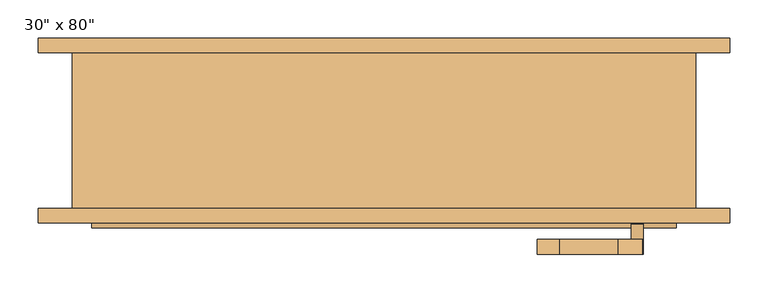
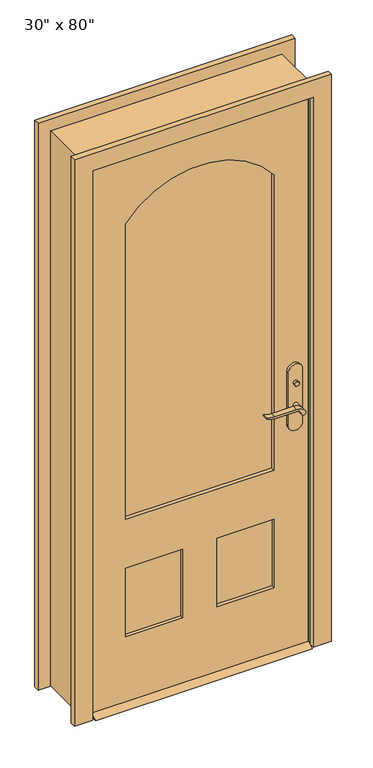
"""IFC4 building model written with IfcOpenShell, lengths in millimetres: door geometry."""

from ifc_helpers import new_model, si_unit, point, frame, frame_2d, origin, place, context, project, spatial, polyline, circle_curve, trimmed, segment, composite_curve, outline, extrude, faceted_brep, source, transform, mapped, element, save


def door_41326d50(model_context):
    return source(origin(), model_context, "Body", "SolidModel", [
        extrude(outline(polyline([(-63.5, 12.7), (-38.1, 0.0), (-123.825, 0.0), (-98.425, 12.7), (-63.5, 12.7)])), frame((-381.0, 0.0, 0.0), z_axis=(1.0, 0.0, 0.0), x_axis=(0.0, 1.0, 0.0)), (0.0, 0.0, 1.0), 762.0),
        extrude(outline(polyline([(335.2, -43.5), (335.2, -53.5), (325.2, -53.5), (325.2, -43.5), (335.2, -43.5)])), frame((0.0, 0.0, 981.9), z_axis=(0.0, 0.0, 1.0), x_axis=(1.0, 0.0, 0.0)), (0.0, 0.0, 1.0), 30.0),
        extrude(outline(composite_curve([segment(trimmed(circle_curve(frame_2d((996.9, 330.2)), 8.0), [point((996.9, 322.2))], [point((996.9, 338.2))], False, "CARTESIAN"), True, "CONTINUOUS"), segment(trimmed(circle_curve(frame_2d((996.9, 330.2)), 8.0), [point((996.9, 338.2))], [point((996.9, 322.2))], False, "CARTESIAN"), True, "CONTINUOUS")], self_intersect=False)), frame((0.0, -118.425, 0.0), z_axis=(0.0, 1.0, 0.0), x_axis=(0.0, 0.0, 1.0)), (0.0, 0.0, 1.0), 10.0),
        extrude(outline(composite_curve([segment(trimmed(circle_curve(frame_2d((897.1555521, 306.5324871)), 37.2832219), [point((919.0523287, 336.7081363))], [point((934.4, 304.8325667))], False, "CARTESIAN"), True, "CONTINUOUS"), segment(polyline([(934.4, 304.8325667), (934.4, 228.5564091)]), True, "CONTINUOUS"), segment(trimmed(circle_curve(frame_2d((1017.6850638, 228.6227909)), 83.2850902), [point((934.4, 228.5564091))], [point((939.4, 200.2))], True, "CARTESIAN"), True, "CONTINUOUS"), segment(polyline([(939.4, 200.2), (936.6135558, 200.2)]), True, "CONTINUOUS"), segment(trimmed(circle_curve(frame_2d((986.6709207, 232.1396612)), 59.3791355), [point((936.6135558, 200.2))], [point((927.4, 228.5564091))], False, "CARTESIAN"), True, "CONTINUOUS"), segment(polyline([(927.4, 228.5564091), (927.4, 304.8138099)]), True, "CONTINUOUS"), segment(trimmed(circle_curve(frame_2d((909.2738613, 304.8138099)), 18.1261387), [point((927.4, 304.8138099))], [point((914.4, 322.2))], True, "CARTESIAN"), True, "CONTINUOUS"), segment(trimmed(circle_curve(frame_2d((914.4, 330.2)), 8.0), [point((914.4, 322.2))], [point((919.0523287, 336.7081363))], False, "CARTESIAN"), True, "CONTINUOUS")], self_intersect=False)), frame((0.0, -23.5, 0.0), z_axis=(0.0, 1.0, 0.0), x_axis=(0.0, 0.0, 1.0)), (0.0, 0.0, 1.0), 20.0),
        extrude(outline(composite_curve([segment(trimmed(circle_curve(frame_2d((914.4, 330.2)), 8.0), [point((914.3999903, 322.2))], [point((919.0523287, 336.7081363))], False, "CARTESIAN"), True, "CONTINUOUS"), segment(trimmed(circle_curve(frame_2d((897.1555521, 306.5324871)), 37.2832219), [point((919.0523287, 336.7081363))], [point((934.4, 304.8325667))], False, "CARTESIAN"), True, "CONTINUOUS"), segment(polyline([(934.4, 304.8325667), (934.4, 228.5564091)]), True, "CONTINUOUS"), segment(trimmed(circle_curve(frame_2d((1017.6850638, 228.6227909)), 83.2850902), [point((934.4, 228.5564091))], [point((939.4, 200.2))], True, "CARTESIAN"), True, "CONTINUOUS"), segment(polyline([(939.4, 200.2), (936.6135558, 200.2)]), True, "CONTINUOUS"), segment(trimmed(circle_curve(frame_2d((986.6709207, 232.1396612)), 59.3791355), [point((936.6135558, 200.2))], [point((927.4, 228.5564091))], False, "CARTESIAN"), True, "CONTINUOUS"), segment(polyline([(927.4, 228.5564091), (927.4, 304.8138122)]), True, "CONTINUOUS"), segment(trimmed(circle_curve(frame_2d((909.2738682, 304.8138122)), 18.1261318), [point((927.4, 304.8138122))], [point((914.3999903, 322.2))], True, "CARTESIAN"), True, "CONTINUOUS")], self_intersect=False)), frame((0.0, -158.425, 0.0), z_axis=(0.0, 1.0, 0.0), x_axis=(0.0, 0.0, 1.0)), (0.0, 0.0, 1.0), 20.0),
        extrude(outline(composite_curve([segment(trimmed(circle_curve(frame_2d((914.4, 330.2)), 8.0), [point((914.4, 322.2))], [point((914.4, 338.2))], False, "CARTESIAN"), True, "CONTINUOUS"), segment(trimmed(circle_curve(frame_2d((914.4, 330.2)), 8.0), [point((914.4, 338.2))], [point((914.4, 322.2))], False, "CARTESIAN"), True, "CONTINUOUS")], self_intersect=False)), frame((0.0, -53.5, 0.0), z_axis=(0.0, 1.0, 0.0), x_axis=(0.0, 0.0, 1.0)), (0.0, 0.0, 1.0), 30.0),
        extrude(outline(composite_curve([segment(trimmed(circle_curve(frame_2d((914.4, 330.2)), 8.0), [point((914.4, 322.2))], [point((914.4, 338.2))], False, "CARTESIAN"), True, "CONTINUOUS"), segment(trimmed(circle_curve(frame_2d((914.4, 330.2)), 8.0), [point((914.4, 338.2))], [point((914.4, 322.2))], False, "CARTESIAN"), True, "CONTINUOUS")], self_intersect=False)), frame((0.0, -138.425, 0.0), z_axis=(0.0, 1.0, 0.0), x_axis=(0.0, 0.0, 1.0)), (0.0, 0.0, 1.0), 30.0),
        extrude(outline(composite_curve([segment(polyline([(844.4, 355.2), (1039.4, 355.2)]), True, "CONTINUOUS"), segment(trimmed(circle_curve(frame_2d((1039.4, 330.2)), 25.0), [point((1039.4, 355.2))], [point((1039.4, 305.2))], False, "CARTESIAN"), True, "CONTINUOUS"), segment(polyline([(1039.4, 305.2), (844.4, 305.2)]), True, "CONTINUOUS"), segment(trimmed(circle_curve(frame_2d((844.4, 330.2)), 25.0), [point((844.4, 305.2))], [point((844.4, 355.2))], False, "CARTESIAN"), True, "CONTINUOUS")], self_intersect=False)), frame((0.0, -63.5, 0.0), z_axis=(0.0, 1.0, 0.0), x_axis=(0.0, 0.0, 1.0)), (0.0, 0.0, 1.0), 10.0),
        extrude(outline(composite_curve([segment(polyline([(844.4, 355.2), (1039.4, 355.2)]), True, "CONTINUOUS"), segment(trimmed(circle_curve(frame_2d((1039.4, 330.2)), 25.0), [point((1039.4, 355.2))], [point((1039.4, 305.2))], False, "CARTESIAN"), True, "CONTINUOUS"), segment(polyline([(1039.4, 305.2), (844.4, 305.2)]), True, "CONTINUOUS"), segment(trimmed(circle_curve(frame_2d((844.4, 330.2)), 25.0), [point((844.4, 305.2))], [point((844.4, 355.2))], False, "CARTESIAN"), True, "CONTINUOUS")], self_intersect=False)), frame((0.0, -108.425, 0.0), z_axis=(0.0, 1.0, 0.0), x_axis=(0.0, 0.0, 1.0)), (0.0, 0.0, 1.0), 10.0),
        extrude(outline(polyline([(2032.0, -381.0), (12.7, -381.0), (12.7, 381.0), (2032.0, 381.0), (2032.0, -381.0)]), holes=[composite_curve([segment(polyline([(688.975, -260.35), (1784.35, -260.35)]), True, "CONTINUOUS"), segment(trimmed(circle_curve(frame_2d((1580.99125, 0.0)), 330.35875), [point((1784.35, -260.35))], [point((1784.35, 260.35))], True, "CARTESIAN"), True, "CONTINUOUS"), segment(polyline([(1784.35, 260.35), (688.975, 260.35), (688.975, -260.35)]), True, "CONTINUOUS")], self_intersect=False), polyline([(508.0, -60.325), (254.0, -60.325), (254.0, -260.35), (508.0, -260.35), (508.0, -60.325)]), polyline([(508.0, 260.35), (254.0, 260.35), (254.0, 60.325), (508.0, 60.325), (508.0, 260.35)])]), frame((0.0, -98.425, 0.0), z_axis=(0.0, 1.0, 0.0), x_axis=(0.0, 0.0, 1.0)), (0.0, 0.0, 1.0), 34.925),
        faceted_brep([(406.4, -98.425, 0.0), (381.0, -98.425, 0.0), (381.0, -63.5, 0.0), (368.3, -63.5, 0.0), (368.3, -28.575, 0.0), (381.0, -28.575, 0.0), (381.0, 104.775, 0.0), (406.4, 104.775, 0.0), (406.4, 104.775, 2057.4), (406.4, -98.425, 2057.4), (381.0, 104.775, 2032.0), (-381.0, 104.775, 2032.0), (-381.0, 104.775, 0.0), (-406.4, 104.775, 0.0), (-406.4, 104.775, 2057.4), (381.0, -28.575, 2032.0), (368.3, -28.575, 2019.3), (-368.3, -28.575, 2019.3), (-368.3, -28.575, 0.0), (-381.0, -28.575, 0.0), (-381.0, -28.575, 2032.0), (368.3, -63.5, 2019.3), (381.0, -63.5, 2032.0), (-381.0, -63.5, 2032.0), (-381.0, -63.5, 0.0), (-368.3, -63.5, 0.0), (-368.3, -63.5, 2019.3), (381.0, -98.425, 2032.0), (-406.4, -98.425, 2057.4), (-406.4, -98.425, 0.0), (-381.0, -98.425, 0.0), (-381.0, -98.425, 2032.0)], [[[0, 1, 2, 3, 4, 5, 6, 7]], [[7, 8, 9, 0]], [[6, 10, 11, 12, 13, 14, 8, 7]], [[5, 15, 10, 6]], [[4, 16, 17, 18, 19, 20, 15, 5]], [[3, 21, 16, 4]], [[2, 22, 23, 24, 25, 26, 21, 3]], [[1, 27, 22, 2]], [[0, 9, 28, 29, 30, 31, 27, 1]], [[8, 14, 28, 9]], [[15, 20, 11, 10]], [[21, 26, 17, 16]], [[27, 31, 23, 22]], [[29, 13, 12, 19, 18, 25, 24, 30]], [[14, 13, 29, 28]], [[20, 19, 12, 11]], [[26, 25, 18, 17]], [[31, 30, 24, 23]]]),
        extrude(outline(polyline([(-60.325, -75.1416667), (-60.325, -86.7833333), (-260.35, -86.7833333), (-260.35, -75.1416667), (-60.325, -75.1416667)])), frame((0.0, 0.0, 254.0), z_axis=(0.0, 0.0, 1.0), x_axis=(1.0, 0.0, 0.0)), (0.0, 0.0, 1.0), 254.0),
        extrude(outline(polyline([(260.35, -75.1416667), (260.35, -86.7833333), (60.325, -86.7833333), (60.325, -75.1416667), (260.35, -75.1416667)])), frame((0.0, 0.0, 254.0), z_axis=(0.0, 0.0, 1.0), x_axis=(1.0, 0.0, 0.0)), (0.0, 0.0, 1.0), 254.0),
        extrude(outline(composite_curve([segment(polyline([(688.975, -260.35), (688.975, 260.35), (1784.35, 260.35)]), True, "CONTINUOUS"), segment(trimmed(circle_curve(frame_2d((1580.99125, 0.0)), 330.35875), [point((1784.35, 260.35))], [point((1784.35, -260.35))], False, "CARTESIAN"), True, "CONTINUOUS"), segment(polyline([(1784.35, -260.35), (688.975, -260.35)]), True, "CONTINUOUS")], self_intersect=False)), frame((0.0, -84.455, 0.0), z_axis=(0.0, 1.0, 0.0), x_axis=(0.0, 0.0, 1.0)), (0.0, 0.0, 1.0), 6.985),
        extrude(outline(polyline([(0.0, -387.35), (2038.35, -387.35), (2038.35, 387.35), (0.0, 387.35), (0.0, 450.85), (2101.85, 450.85), (2101.85, -450.85), (0.0, -450.85), (0.0, -387.35)])), frame((0.0, 104.775, 0.0), z_axis=(0.0, 1.0, 0.0), x_axis=(0.0, 0.0, 1.0)), (0.0, 0.0, 1.0), 19.05),
        extrude(outline(polyline([(0.0, -387.35), (2038.35, -387.35), (2038.35, 387.35), (0.0, 387.35), (0.0, 450.85), (2101.85, 450.85), (2101.85, -450.85), (0.0, -450.85), (0.0, -387.35)])), frame((0.0, -117.475, 0.0), z_axis=(0.0, 1.0, 0.0), x_axis=(0.0, 0.0, 1.0)), (0.0, 0.0, 1.0), 19.05),
    ])


if __name__ == "__main__":
    model = new_model("IFC4")
    model_context = context("Model", 3, world=origin())
    ifc_project = project(units=[si_unit("LENGTHUNIT", "METRE", prefix="MILLI")], contexts=[model_context])
    site = spatial("IfcSite", under=ifc_project)
    building = spatial("IfcBuilding", under=site)
    placement = place(None, origin())
    door_shape = door_41326d50(model_context)
    element("IfcDoor", 1, ObjectType="30\" x 80\"", at=placement, inside=building, context=model_context, shape_type="MappedRepresentation", body=[
        mapped(door_shape, transform((0.0, 0.0, 0.0), x_axis=(1.0, 0.0, 0.0), y_axis=(0.0, 1.0, 0.0), z_axis=(0.0, 0.0, 1.0))),
    ])
    save(model, "model.ifc")

# Revit data of these elements
# Type "30\" x 80\""
#   Type Mark = "8"
#   Assembly Code = "B2030100"
#   Analytic Construction = "French door, wood frame with single glass"
#   Threshold Offset [instance default] = 0' - 0 1/2"
#   Thickness = 0' - 1 3/8"
#   Thermal Resistance (R) = 1.0696 (h·ft²·°F)/BTU
#   Swing Angle [instance default] = 90.00°
#   Stiles = 0' - 4 3/4"
#   Rough Width = 2' - 8"
#   Rough Height = 6' - 9"
#   Radius = 1' - 1.00625"
#   Lock Rail = 0' - 7 1/8"
#   Height = 6' - 8"
#   Width = 2' - 6"
#   Heat Transfer Coefficient (U) = 0.9350 BTU/(h·ft²·°F)
#   Door Offset [instance default] = 0' - 0"
#   Bottom Rail = 0' - 9 1/2"
#   Threshold [instance default] = yes
#   Function = 1
#   Exterior Trim [instance default] = yes
#   Trim Material = Cherry
#   Threshold Material = Cherry
#   Panel Material = Cherry
#   Glazing = Glass
#   Frame Material = Cherry
#   Door Handle Material = Aluminum
#   Visual Light Transmittance = 0
#   Solar Heat Gain Coefficient = 0
#   Wall Closure = (empty or 0)
#   Construction Type = (empty or 0)
# Element 1 (IfcDoor, "30\" x 80\"")
#   Materials on its faces: "Cherry", "Aluminum", "Glass"
# Materials
#   "Cherry": class "Wood", colour RGB 226 177 128, transparency 0, Description = "Prunus Serotina", Cost = 0
#   "Glass": class "Glass", colour RGB 0 128 192, transparency 0.75, Description = "Soda Lime Glass", Cost = 0
#   "Aluminum": class "Metal", colour RGB 247 247 247, transparency 0, Description = "Aluminum 6061", Cost = 0
